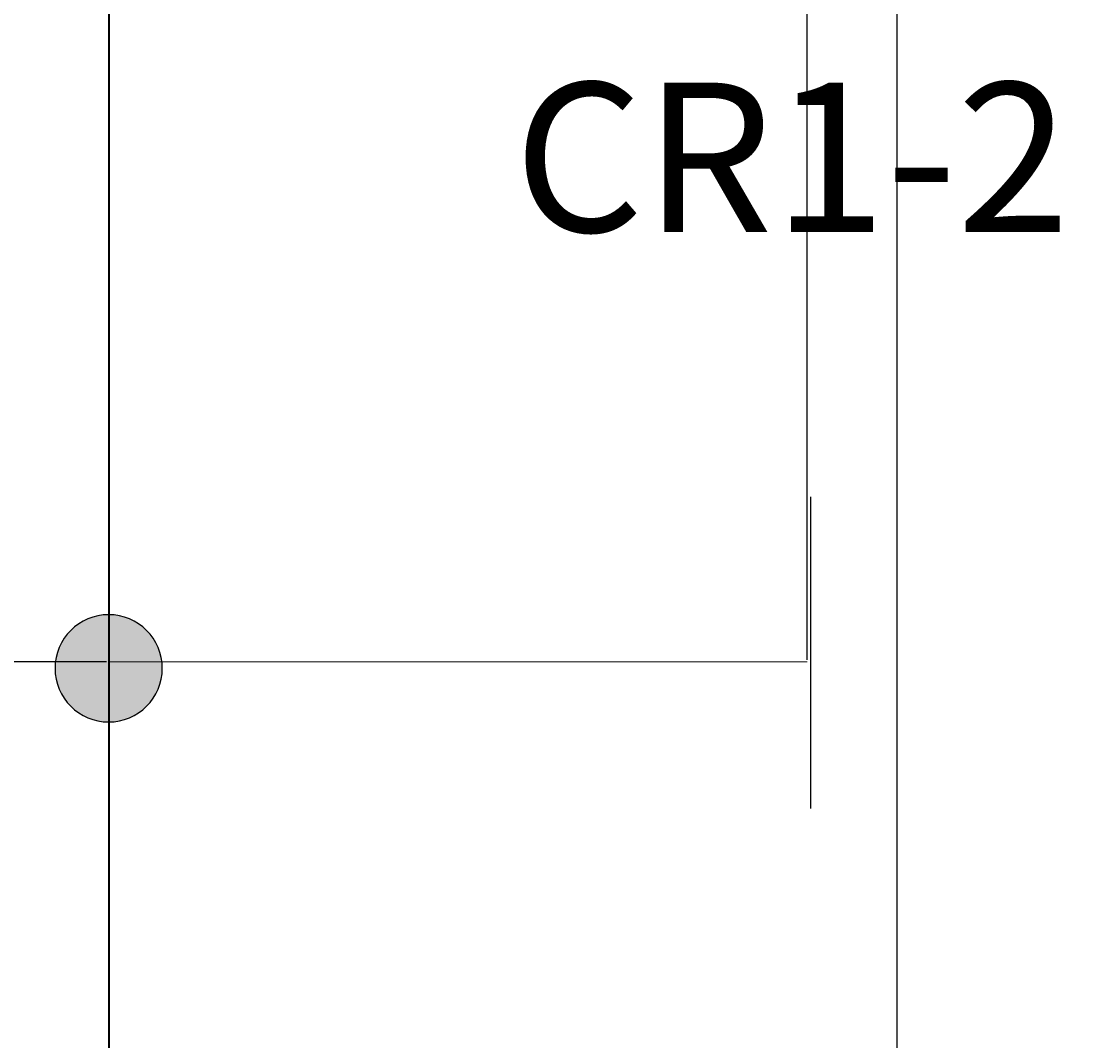
# Model space of a CAD drawing. Units: inches. Extents: x 738 to 1068, y 378 to 757.
# Tile 21 of 41: x 779 to 809, y 521 to 549. Entities that reach past the tile are written whole.
import ezdxf

# ---------------------------------------------------------------- set-up
doc = ezdxf.new("R2010")
doc.units = ezdxf.units.IN
doc.header["$MEASUREMENT"] = 0
for name, color, linetype, lineweight in [('A-ANNO-DIMS', 2, 'Continuous', 18), ('E-ANNO-TEXT', 7, 'Continuous', 18), ('E-CONN', 7, 'Continuous', 25), ('E-CTRL-CONT', 4, 'Continuous', 25), ('E-CTRL-WIRE', 7, 'Continuous', 18), ('E-POWR-FEED', 7, 'Continuous', 35)]:
    doc.layers.add(name, color=color, linetype=linetype, lineweight=lineweight)
doc.styles.get("Standard").update_dxf_attribs({"font": 'arial.ttf'})
doc.dimstyles.get("Standard").update_dxf_attribs({"dimtxt": 0.18, "dimasz": 0.18, "dimexe": 0.18, "dimexo": 0.0625, "dimgap": 0.09, "dimtad": 0, "dimtih": 1, "dimtoh": 1, "dimdec": 4, "dimzin": 0, "dimdsep": 46, "dimtxsty": 'Standard', "dimcen": 0.09, "dimadec": 0, "dimazin": 0, "dimtfac": 1, "dimtdec": 4, "dimtofl": 0, "dimtmove": 0, "dimatfit": 3, "dimfxl": 1, "dimtolj": 1, "dimtzin": 0, "dimarcsym": 0})

# ---------------------------------------------------------------- blocks, each defined once
blk = doc.blocks.new('CR-AUX-CONTACT-NO')
for p, q in [((0, 8.72), (0, 0)), ((8.265, 8.72), (8.265, 0))]:
    blk.add_line(p, q)
blk = doc.blocks.new('RUNG-JUNCTION')
h = blk.add_hatch(color=256)
h.dxf.hatch_style = 1
h.paths.add_polyline_path([(3, 1.5, 1), (0, 1.5, 1)])
blk.add_lwpolyline([(0, 1.5, 1), (3, 1.5, 1)], format="xyb", close=True)
blk = doc.blocks.new('*D21')
at = {"layer": 'A-ANNO-DIMS', "color": 0, "lineweight": -2, "transparency": 16777216}
for p, q in [((781.427, 531.401), (738.194, 531.401)), ((738.374, 531.221), (738.374, 496.578)), ((738.374, 461.572), (738.374, 496.215)), ((781.427, 461.392), (738.194, 461.392))]:
    blk.add_line(p, q, dxfattribs=at)
at = {"layer": 'A-ANNO-DIMS', "color": 0, "transparency": 16777216}
for points in [[(738.344, 531.221), (738.404, 531.221), (738.374, 531.401)], [(738.344, 461.572), (738.404, 461.572), (738.374, 461.392)]]:
    blk.add_solid(points, dxfattribs=at)
at = {"layer": 'Defpoints', "color": 0, "transparency": 16777216}
for p in [(738.374, 531.401), (781.49, 531.401), (781.49, 461.392)]:
    blk.add_point(p, dxfattribs=at)
at = {"layer": 'A-ANNO-DIMS', "color": 0, "transparency": 16777216, "insert": (738.374, 496.396), "char_height": 0.18, "attachment_point": 5}
blk.add_mtext('\\A1;70.01', dxfattribs=at)
blk = doc.blocks.new('*D22')
at = {"layer": 'A-ANNO-DIMS', "color": 0, "lineweight": -2, "transparency": 16777216}
for p, q in [((781.422, 593.08), (738.194, 593.08)), ((738.374, 592.9), (738.374, 562.422)), ((738.374, 531.581), (738.374, 562.058)), ((781.427, 531.401), (738.194, 531.401))]:
    blk.add_line(p, q, dxfattribs=at)
at = {"layer": 'A-ANNO-DIMS', "color": 0, "transparency": 16777216}
for points in [[(738.344, 592.9), (738.404, 592.9), (738.374, 593.08)], [(738.344, 531.581), (738.404, 531.581), (738.374, 531.401)]]:
    blk.add_solid(points, dxfattribs=at)
at = {"layer": 'Defpoints', "color": 0, "transparency": 16777216}
for p in [(738.374, 593.08), (781.485, 593.08), (781.49, 531.401)]:
    blk.add_point(p, dxfattribs=at)
at = {"layer": 'A-ANNO-DIMS', "color": 0, "transparency": 16777216, "insert": (738.374, 562.24), "char_height": 0.18, "attachment_point": 5}
blk.add_mtext('\\A1;61.68', dxfattribs=at)
blk = doc.blocks.new('*D25')
at = {"layer": 'A-ANNO-DIMS', "color": 0, "lineweight": -2, "transparency": 16777216}
for p, q in [((781.49, 646.923), (781.49, 378.239)), ((803.522, 646.923), (803.522, 378.239)), ((781.67, 378.419), (792.111, 378.419)), ((803.342, 378.419), (792.901, 378.419))]:
    blk.add_line(p, q, dxfattribs=at)
at = {"layer": 'A-ANNO-DIMS', "color": 0, "transparency": 16777216}
for points in [[(781.67, 378.449), (781.67, 378.389), (781.49, 378.419)], [(803.342, 378.449), (803.342, 378.389), (803.522, 378.419)]]:
    blk.add_solid(points, dxfattribs=at)
at = {"layer": 'Defpoints', "color": 0, "transparency": 16777216}
for p in [(781.49, 646.985), (803.522, 646.985), (803.522, 378.419)]:
    blk.add_point(p, dxfattribs=at)
at = {"layer": 'A-ANNO-DIMS', "color": 0, "transparency": 16777216, "insert": (792.506, 378.419), "char_height": 0.18, "attachment_point": 5}
blk.add_mtext('\\A1;22.03', dxfattribs=at)
blk = doc.blocks.new('*D31')
at = {"layer": 'A-ANNO-DIMS', "color": 0, "lineweight": -2, "transparency": 16777216}
for p, q in [((781.49, 531.463), (781.49, 756.505)), ((781.67, 756.325), (790.802, 756.325)), ((800.842, 756.325), (791.71, 756.325)), ((801.022, 531.463), (801.022, 756.505))]:
    blk.add_line(p, q, dxfattribs=at)
at = {"layer": 'A-ANNO-DIMS', "color": 0, "transparency": 16777216}
for points in [[(781.67, 756.355), (781.67, 756.295), (781.49, 756.325)], [(800.842, 756.355), (800.842, 756.295), (801.022, 756.325)]]:
    blk.add_solid(points, dxfattribs=at)
at = {"layer": 'Defpoints', "color": 0, "transparency": 16777216}
for p in [(801.022, 756.325), (781.49, 531.401), (801.022, 531.401)]:
    blk.add_point(p, dxfattribs=at)
at = {"layer": 'A-ANNO-DIMS', "color": 0, "transparency": 16777216, "insert": (791.256, 756.325), "char_height": 0.18, "attachment_point": 5}
blk.add_mtext('\\A1;19.532', dxfattribs=at)
blk = doc.blocks.new('*D34')
at = {"layer": 'A-ANNO-DIMS', "color": 0, "lineweight": -2, "transparency": 16777216}
for p, q in [((781.49, 686.266), (781.49, 378.239)), ((830.489, 686.266), (830.489, 378.239)), ((781.67, 378.419), (805.767, 378.419)), ((830.309, 378.419), (806.212, 378.419))]:
    blk.add_line(p, q, dxfattribs=at)
at = {"layer": 'A-ANNO-DIMS', "color": 0, "transparency": 16777216}
for points in [[(781.67, 378.449), (781.67, 378.389), (781.49, 378.419)], [(830.309, 378.449), (830.309, 378.389), (830.489, 378.419)]]:
    blk.add_solid(points, dxfattribs=at)
at = {"layer": 'Defpoints', "color": 0, "transparency": 16777216}
for p in [(781.49, 686.329), (830.489, 686.329), (830.489, 378.419)]:
    blk.add_point(p, dxfattribs=at)
at = {"layer": 'A-ANNO-DIMS', "color": 0, "transparency": 16777216, "insert": (805.99, 378.419), "char_height": 0.18, "attachment_point": 5}
blk.add_mtext('\\A1;49', dxfattribs=at)
blk = doc.blocks.new('*D38')
at = {"layer": 'A-ANNO-DIMS', "color": 0, "lineweight": -2, "transparency": 16777216}
for p, q in [((781.485, 593.017), (781.485, 378.239)), ((887.04, 593.067), (887.04, 378.239)), ((781.665, 378.419), (833.807, 378.419)), ((886.86, 378.419), (834.718, 378.419))]:
    blk.add_line(p, q, dxfattribs=at)
at = {"layer": 'A-ANNO-DIMS', "color": 0, "transparency": 16777216}
for points in [[(781.665, 378.449), (781.665, 378.389), (781.485, 378.419)], [(886.86, 378.449), (886.86, 378.389), (887.04, 378.419)]]:
    blk.add_solid(points, dxfattribs=at)
at = {"layer": 'Defpoints', "color": 0, "transparency": 16777216}
for p in [(781.485, 593.08), (887.04, 593.13), (887.04, 378.419)]:
    blk.add_point(p, dxfattribs=at)
at = {"layer": 'A-ANNO-DIMS', "color": 0, "transparency": 16777216, "insert": (834.263, 378.419), "char_height": 0.18, "attachment_point": 5}
blk.add_mtext('\\A1;105.56', dxfattribs=at)

msp = doc.modelspace()

# ---------------------------------------------------------------- linework, layer by layer
at = {"layer": 'E-CTRL-WIRE'}
msp.add_line((781.4897, 531.4009), (801.0218, 531.4009), dxfattribs=at)
at = {"layer": 'E-POWR-FEED'}
msp.add_line((781.4897, 686.329), (781.4897, 437.7164), dxfattribs=at)

# ---------------------------------------------------------------- block references
at = {"layer": 'E-CONN'}
msp.add_blockref('RUNG-JUNCTION', (779.985, 529.7226), dxfattribs=at)
at = {"layer": 'E-CTRL-CONT'}
msp.add_blockref('CR-AUX-CONTACT-NO', (801.115, 527.299), dxfattribs=at)

# ---------------------------------------------------------------- texts
at = {"layer": 'E-ANNO-TEXT'}
msp.add_text('CR1-2', height=4.17507, dxfattribs=at).set_placement((792.8126, 543.4263))

# ---------------------------------------------------------------- dimensions: what is measured, and where the dimension line sits
at = {"layer": 'A-ANNO-DIMS'}
for base, p1, p2, override, picture, middle in [((801.0218, 756.3251), (781.4897, 531.4009), (801.0218, 531.4009), {"dimdec": 3, "dimlfac": 1, "dimrnd": 0, "dimzin": 0, "dimdsep": 46, "dimlunit": 2}, '*D31', (791.2557, 756.3251)), ((830.4893, 378.4191), (781.4897, 686.329), (830.4893, 686.329), {"dimdec": 0, "dimlfac": 1, "dimrnd": 0, "dimzin": 0, "dimdsep": 46, "dimlunit": 2}, '*D34', (805.9895, 378.4191)), ((803.5218, 378.4191), (781.4897, 646.9853), (803.5218, 646.9853), {"dimdec": 2, "dimlfac": 1, "dimrnd": 0, "dimzin": 0, "dimdsep": 46, "dimlunit": 2}, '*D25', (792.5057, 378.4191)), ((887.0404, 378.4191), (781.4846, 593.0796), (887.0404, 593.1296), {"dimdec": 2, "dimlfac": 1, "dimrnd": 0, "dimzin": 0, "dimdsep": 46, "dimlunit": 2}, '*D38', (834.2625, 378.4191))]:
    dim = msp.add_linear_dim(base=base, p1=p1, p2=p2, dimstyle='Standard', override=override, dxfattribs=at)
    dim.commit()
    dim.dimension.update_dxf_attribs({"geometry": picture, "text_midpoint": middle})
for base, p1, p2, picture, middle in [((738.3736, 593.0796), (781.4897, 531.4009), (781.4846, 593.0796), '*D22', (738.3736, 562.2403)), ((738.3736, 531.4009), (781.4897, 461.3919), (781.4897, 531.4009), '*D21', (738.3736, 496.3964))]:
    dim = msp.add_linear_dim(base=base, p1=p1, p2=p2, angle=90, dimstyle='Standard', override={"dimdec": 2, "dimlfac": 1, "dimrnd": 0, "dimzin": 0, "dimdsep": 46, "dimlunit": 2}, dxfattribs=at)
    dim.commit()
    dim.dimension.update_dxf_attribs({"geometry": picture, "text_midpoint": middle})

doc.saveas('drawing.dxf')
